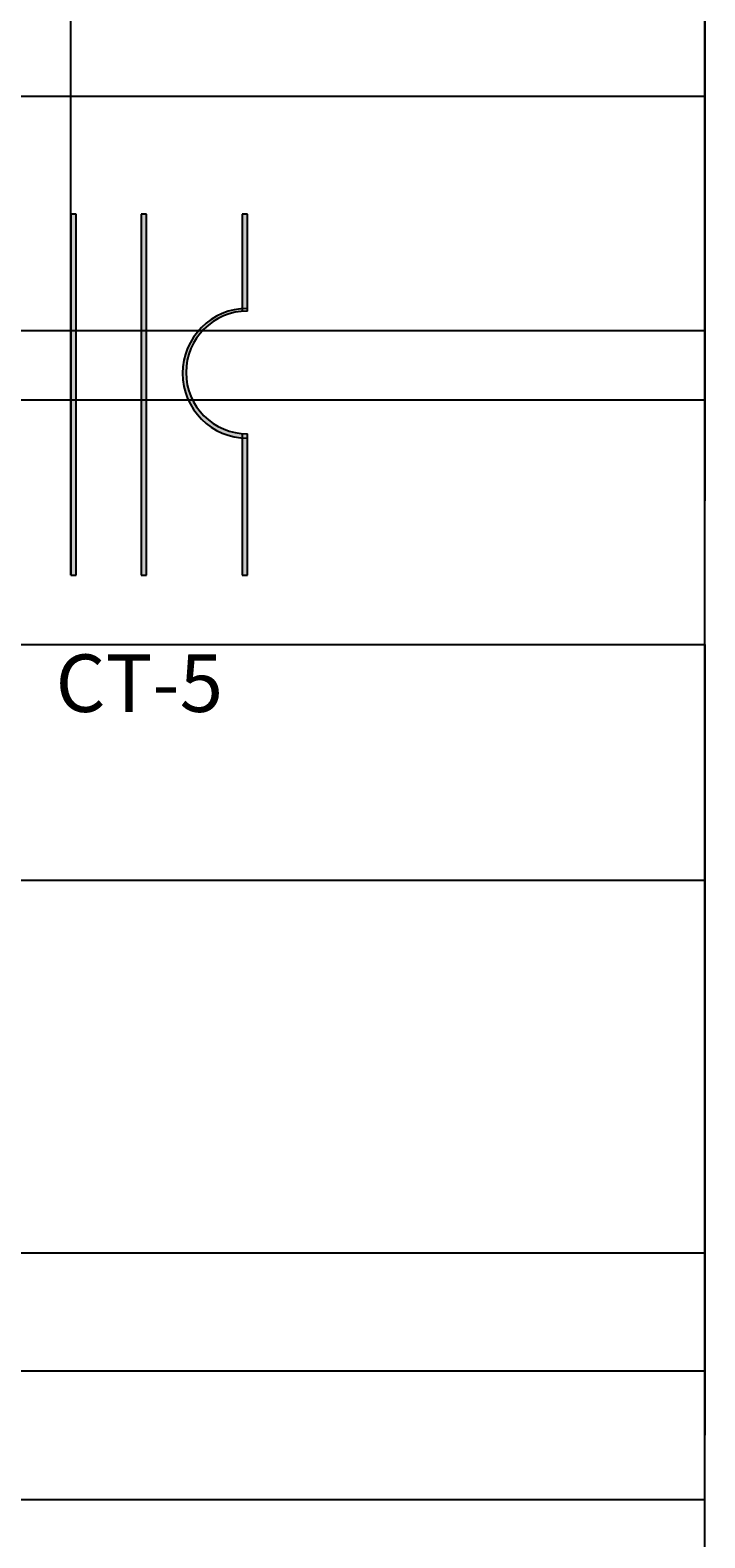
# Model space of a CAD drawing. Units: inches. Extents: x 35362 to 73946, y 43607 to 67532.
# Tile 134 of 134: x 71350 to 73946, y 55752 to 61547. Entities that reach past the tile are written whole.
import ezdxf

# ---------------------------------------------------------------- set-up
doc = ezdxf.new("R2010")
doc.units = ezdxf.units.IN
doc.header["$MEASUREMENT"] = 0
for name, color, linetype, lineweight in [('A-ANNO-DIMS', 2, 'Continuous', 18), ('E-ANNO-TEXT', 5, 'Continuous', 18), ('E-SYMB', 1, 'Continuous', 25), ('E-SYMB-PATT', 1, 'Continuous', 13)]:
    doc.layers.add(name, color=color, linetype=linetype, lineweight=lineweight)
doc.styles.get("Standard").update_dxf_attribs({"font": 'arial.ttf'})
doc.dimstyles.get("Standard").update_dxf_attribs({"dimtxt": 0.18, "dimasz": 0.18, "dimexe": 0.18, "dimexo": 0.0625, "dimgap": 0.09, "dimtad": 0, "dimtih": 1, "dimtoh": 1, "dimdec": 4, "dimzin": 0, "dimdsep": 46, "dimtxsty": 'Standard', "dimcen": 0.09, "dimadec": 0, "dimazin": 0, "dimtfac": 1, "dimtdec": 4, "dimtofl": 0, "dimtmove": 0, "dimatfit": 3, "dimfxl": 1, "dimtolj": 1, "dimtzin": 0, "dimarcsym": 0})

# ---------------------------------------------------------------- blocks, each defined once
blk = doc.blocks.new('CT-CORE')
for p, q in [((-0.0004610742907971, 1387.996120092102), (-0.0004610742907971, -5.34733626409e-05)), ((19.99953892572375, 1387.996120092102), (-0.0004610742907971, 1387.996120092102)), ((19.9995389257092, -5.34733626409e-05), (19.99953892572375, 1387.996120092102)), ((270.6681283192447, 1387.996120092102), (270.6681283192447, -5.34733626409e-05)), ((290.6681283192593, 1387.996120092102), (270.6681283192447, 1387.996120092102)), ((290.6681283192447, -5.34733626409e-05), (290.6681283192593, 1387.996120092102)), ((658.9826659540267, 1387.996120092102), (658.9826659540267, 1014.585417332389)), ((678.9826659540413, 1387.996120092102), (658.9826659540267, 1387.996120092102)), ((678.9826659540413, 1015.434583844784), (678.9826659540413, 1387.996120092102)), ((658.9826659540267, 544.3844491987692), (658.9826659540267, -5.34733626409e-05)), ((678.9826659540267, -5.34733626409e-05), (678.9826659540413, 543.5352826863744)), ((-0.0004610742907971, -5.34733626409e-05), (19.9995389257092, -5.34733626409e-05)), ((270.6681283192447, -5.34733626409e-05), (290.6681283192447, -5.34733626409e-05)), ((658.9826659540267, -5.34733626409e-05), (678.9826659540267, -5.34733626409e-05))]:
    blk.add_line(p, q)
blk.add_arc((678.9826659540267, 779.4849332655793), 235.9496505792049, 90, 270)
blk = doc.blocks.new('*D8')
at = {"layer": 'A-ANNO-DIMS', "color": 0, "lineweight": -2, "transparency": 16777216}
for p, q in [((66271.28651900003, 65771.51172800003), (73945.82566600003, 65771.51172800003)), ((73945.64566600005, 65771.33172800003), (73945.64566600005, 59737.03093663782)), ((73945.64566600005, 53702.36633900002), (73945.64566600005, 59736.66713036224)), ((72185.70816600003, 53702.18633900003), (73945.82566600003, 53702.18633900003))]:
    blk.add_line(p, q, dxfattribs=at)
at = {"layer": 'A-ANNO-DIMS', "color": 0, "transparency": 16777216}
for points in [[(73945.61566600006, 65771.33172800003), (73945.67566600005, 65771.33172800003), (73945.64566600005, 65771.51172800003)], [(73945.61566600006, 53702.36633900002), (73945.67566600005, 53702.36633900002), (73945.64566600005, 53702.18633900003)]]:
    blk.add_solid(points, dxfattribs=at)
at = {"layer": 'Defpoints', "color": 0, "transparency": 16777216}
for p in [(66271.22401900003, 65771.51172800003), (73945.64566600005, 65771.51172800003), (72185.64566600003, 53702.18633900003)]:
    blk.add_point(p, dxfattribs=at)
at = {"layer": 'A-ANNO-DIMS', "color": 0, "transparency": 16777216, "insert": (73945.64566600005, 59736.84903349999), "char_height": 0.18, "attachment_point": 5}
blk.add_mtext('\\A1;12069', dxfattribs=at)
blk = doc.blocks.new('*D10')
at = {"layer": 'A-ANNO-DIMS', "color": 0, "lineweight": -2, "transparency": 16777216}
for p, q in [((61240.96983600002, 59185.14395700003), (73945.82566600003, 59185.14395700003)), ((73945.64566600005, 59184.96395700003), (73945.64566600005, 56268.51827402935)), ((73945.64566600005, 53351.70866200003), (73945.64566600005, 56268.1543449707)), ((61240.96983600002, 53351.52866200003), (73945.82566600003, 53351.52866200003))]:
    blk.add_line(p, q, dxfattribs=at)
at = {"layer": 'A-ANNO-DIMS', "color": 0, "transparency": 16777216}
for points in [[(73945.61566600006, 59184.96395700003), (73945.67566600005, 59184.96395700003), (73945.64566600005, 59185.14395700003)], [(73945.61566600006, 53351.70866200003), (73945.67566600005, 53351.70866200003), (73945.64566600005, 53351.52866200003)]]:
    blk.add_solid(points, dxfattribs=at)
at = {"layer": 'Defpoints', "color": 0, "transparency": 16777216}
for p in [(61240.90733600002, 59185.14395700003), (61240.90733600002, 53351.52866200003), (73945.64566600005, 53351.52866200003)]:
    blk.add_point(p, dxfattribs=at)
at = {"layer": 'A-ANNO-DIMS', "color": 0, "transparency": 16777216, "insert": (73945.64566600005, 56268.33630949999), "char_height": 0.18, "attachment_point": 5}
blk.add_mtext('\\A1;5834', dxfattribs=at)
blk = doc.blocks.new('*D47')
at = {"layer": 'A-ANNO-DIMS', "color": 0, "lineweight": -2, "transparency": 16777216}
for p, q in [((50339.58680000003, 58279.98849500002), (73945.82566600003, 58279.98849500002)), ((73945.64566600005, 58279.80849500002), (73945.64566600005, 57564.17141502935)), ((73945.64566600005, 56848.17040600003), (73945.64566600005, 57563.80748597069)), ((50339.58680000003, 56847.99040600003), (73945.82566600003, 56847.99040600003))]:
    blk.add_line(p, q, dxfattribs=at)
at = {"layer": 'A-ANNO-DIMS', "color": 0, "transparency": 16777216}
for points in [[(73945.61566600006, 58279.80849500002), (73945.67566600005, 58279.80849500002), (73945.64566600005, 58279.98849500002)], [(73945.61566600006, 56848.17040600003), (73945.67566600005, 56848.17040600003), (73945.64566600005, 56847.99040600003)]]:
    blk.add_solid(points, dxfattribs=at)
at = {"layer": 'Defpoints', "color": 0, "transparency": 16777216}
for p in [(50339.52430000002, 58279.98849500002), (50339.52430000002, 56847.99040600003), (73945.64566600005, 56847.99040600003)]:
    blk.add_point(p, dxfattribs=at)
at = {"layer": 'A-ANNO-DIMS', "color": 0, "transparency": 16777216, "insert": (73945.64566600005, 57563.98945049999), "char_height": 0.18, "attachment_point": 5}
blk.add_mtext('\\A1;1432.0', dxfattribs=at)
blk = doc.blocks.new('*D50')
at = {"layer": 'A-ANNO-DIMS', "color": 0, "lineweight": -2, "transparency": 16777216}
for p, q in [((61657.28213900003, 56394.41825000003), (73945.82566600003, 56394.41825000003)), ((73945.64566600005, 56394.23825000003), (73945.64566600005, 56147.19337413782)), ((73945.64566600005, 55899.78469200003), (73945.64566600005, 56146.82956786224)), ((61657.28213900003, 55899.60469200002), (73945.82566600003, 55899.60469200002))]:
    blk.add_line(p, q, dxfattribs=at)
at = {"layer": 'A-ANNO-DIMS', "color": 0, "transparency": 16777216}
for points in [[(73945.61566600006, 56394.23825000003), (73945.67566600005, 56394.23825000003), (73945.64566600005, 56394.41825000003)], [(73945.61566600006, 55899.78469200003), (73945.67566600005, 55899.78469200003), (73945.64566600005, 55899.60469200002)]]:
    blk.add_solid(points, dxfattribs=at)
at = {"layer": 'Defpoints', "color": 0, "transparency": 16777216}
for p in [(61657.21963900003, 56394.41825000003), (61657.21963900003, 55899.60469200002), (73945.64566600005, 55899.60469200002)]:
    blk.add_point(p, dxfattribs=at)
at = {"layer": 'A-ANNO-DIMS', "color": 0, "transparency": 16777216, "insert": (73945.64566600005, 56147.01147099999), "char_height": 0.18, "attachment_point": 5}
blk.add_mtext('\\A1;494.8', dxfattribs=at)
blk = doc.blocks.new('*D66')
at = {"layer": 'A-ANNO-DIMS', "color": 0, "lineweight": -2, "transparency": 16777216}
for p, q in [((67326.70224100004, 64127.44160800003), (73945.82566600003, 64127.44160800003)), ((73945.64566600005, 64127.26160800003), (73945.64566600005, 62710.54579452936)), ((73945.64566600005, 61293.46605200003), (73945.64566600005, 62710.1818654707)), ((67326.70224100004, 61293.28605200003), (73945.82566600003, 61293.28605200003))]:
    blk.add_line(p, q, dxfattribs=at)
at = {"layer": 'A-ANNO-DIMS', "color": 0, "transparency": 16777216}
for points in [[(73945.61566600006, 64127.26160800003), (73945.67566600005, 64127.26160800003), (73945.64566600005, 64127.44160800003)], [(73945.61566600006, 61293.46605200003), (73945.67566600005, 61293.46605200003), (73945.64566600005, 61293.28605200003)]]:
    blk.add_solid(points, dxfattribs=at)
at = {"layer": 'Defpoints', "color": 0, "transparency": 16777216}
for p in [(67326.63974100004, 64127.44160800003), (73945.64566600005, 64127.44160800003), (67326.63974100004, 61293.28605200003)]:
    blk.add_point(p, dxfattribs=at)
at = {"layer": 'A-ANNO-DIMS', "color": 0, "transparency": 16777216, "insert": (73945.64566600005, 62710.36383), "char_height": 0.18, "attachment_point": 5}
blk.add_mtext('\\A1;2834.2', dxfattribs=at)
blk = doc.blocks.new('*D69')
at = {"layer": 'A-ANNO-DIMS', "color": 0, "lineweight": -2, "transparency": 16777216}
for p, q in [((68320.870762, 60122.408832), (68320.870762, 67531.691728)), ((68321.050762, 67531.51172799998), (69913.30289879469, 67531.51172799998)), ((71506.482539, 67531.51172799998), (69914.23040220531, 67531.51172799998)), ((71506.662539, 59451.647447), (71506.662539, 67531.691728))]:
    blk.add_line(p, q, dxfattribs=at)
at = {"layer": 'A-ANNO-DIMS', "color": 0, "transparency": 16777216}
for points in [[(68321.050762, 67531.541728), (68321.050762, 67531.481728), (68320.870762, 67531.51172799998)], [(71506.482539, 67531.541728), (71506.482539, 67531.481728), (71506.662539, 67531.51172799998)]]:
    blk.add_solid(points, dxfattribs=at)
at = {"layer": 'Defpoints', "color": 0, "transparency": 16777216}
for p in [(71506.662539, 67531.51172799998), (68320.870762, 60122.346332), (71506.662539, 59451.584947)]:
    blk.add_point(p, dxfattribs=at)
at = {"layer": 'A-ANNO-DIMS', "color": 0, "transparency": 16777216, "insert": (69913.76665050001, 67531.51172799998), "char_height": 0.18, "attachment_point": 5}
blk.add_mtext('\\A1;3185.8', dxfattribs=at)
blk = doc.blocks.new('*D70')
at = {"layer": 'A-ANNO-DIMS', "color": 0, "lineweight": -2, "transparency": 16777216}
for p, q in [((60785.27513900002, 64923.75242000003), (73945.82566600003, 64923.75242000003)), ((73945.64566600005, 64923.57242000003), (73945.64566600005, 62054.63015302935)), ((73945.64566600005, 59185.32395700003), (73945.64566600005, 62054.26622397069)), ((61240.96983600002, 59185.14395700003), (73945.82566600003, 59185.14395700003))]:
    blk.add_line(p, q, dxfattribs=at)
at = {"layer": 'A-ANNO-DIMS', "color": 0, "transparency": 16777216}
for points in [[(73945.61566600006, 64923.57242000003), (73945.67566600005, 64923.57242000003), (73945.64566600005, 64923.75242000003)], [(73945.61566600006, 59185.32395700003), (73945.67566600005, 59185.32395700003), (73945.64566600005, 59185.14395700003)]]:
    blk.add_solid(points, dxfattribs=at)
at = {"layer": 'Defpoints', "color": 0, "transparency": 16777216}
for p in [(60785.21263900002, 64923.75242000003), (73945.64566600005, 64923.75242000003), (61240.90733600002, 59185.14395700003)]:
    blk.add_point(p, dxfattribs=at)
at = {"layer": 'A-ANNO-DIMS', "color": 0, "transparency": 16777216, "insert": (73945.64566600005, 62054.44818849999), "char_height": 0.18, "attachment_point": 5}
blk.add_mtext('\\A1;5738.6', dxfattribs=at)
blk = doc.blocks.new('*D71')
at = {"layer": 'A-ANNO-DIMS', "color": 0, "lineweight": -2, "transparency": 16777216}
for p, q in [((63159.24181700003, 64828.55626700002), (73945.82566600003, 64828.55626700002)), ((73945.64566600005, 64828.37626700002), (73945.64566600005, 62007.03207652936)), ((73945.64566600005, 59185.32395700003), (73945.64566600005, 62006.6681474707)), ((61240.96983600002, 59185.14395700003), (73945.82566600003, 59185.14395700003))]:
    blk.add_line(p, q, dxfattribs=at)
at = {"layer": 'A-ANNO-DIMS', "color": 0, "transparency": 16777216}
for points in [[(73945.61566600006, 64828.37626700002), (73945.67566600005, 64828.37626700002), (73945.64566600005, 64828.55626700002)], [(73945.61566600006, 59185.32395700003), (73945.67566600005, 59185.32395700003), (73945.64566600005, 59185.14395700003)]]:
    blk.add_solid(points, dxfattribs=at)
at = {"layer": 'Defpoints', "color": 0, "transparency": 16777216}
for p in [(63159.17931700003, 64828.55626700002), (73945.64566600005, 64828.55626700002), (61240.90733600002, 59185.14395700003)]:
    blk.add_point(p, dxfattribs=at)
at = {"layer": 'A-ANNO-DIMS', "color": 0, "transparency": 16777216, "insert": (73945.64566600005, 62006.85011199999), "char_height": 0.18, "attachment_point": 5}
blk.add_mtext('\\A1;5643.4', dxfattribs=at)
blk = doc.blocks.new('*D113')
at = {"layer": 'A-ANNO-DIMS', "color": 0, "lineweight": -2, "transparency": 16777216}
for p, q in [((53526.13474100003, 60391.71935800003), (73945.82566600003, 60391.71935800003)), ((73945.64566600005, 60391.53935800003), (73945.64566600005, 60259.19182863781)), ((73945.64566600005, 60126.48049300003), (73945.64566600005, 60258.82802236224)), ((53705.42262200003, 60126.30049300003), (73945.82566600003, 60126.30049300003))]:
    blk.add_line(p, q, dxfattribs=at)
at = {"layer": 'A-ANNO-DIMS', "color": 0, "transparency": 16777216}
for points in [[(73945.61566600006, 60391.53935800003), (73945.67566600005, 60391.53935800003), (73945.64566600005, 60391.71935800003)], [(73945.61566600006, 60126.48049300003), (73945.67566600005, 60126.48049300003), (73945.64566600005, 60126.30049300003)]]:
    blk.add_solid(points, dxfattribs=at)
at = {"layer": 'Defpoints', "color": 0, "transparency": 16777216}
for p in [(53526.07224100003, 60391.71935800003), (73945.64566600005, 60391.71935800003), (53705.36012200003, 60126.30049300003)]:
    blk.add_point(p, dxfattribs=at)
at = {"layer": 'A-ANNO-DIMS', "color": 0, "transparency": 16777216, "insert": (73945.64566600005, 60259.00992549999), "char_height": 0.18, "attachment_point": 5}
blk.add_mtext('\\A1;265.4', dxfattribs=at)

msp = doc.modelspace()

# ---------------------------------------------------------------- hatches: boundary and pattern name
at = {"layer": 'E-SYMB-PATT'}
h = msp.add_hatch(color=256, dxfattribs=at)
h.dxf.hatch_style = 1
h.paths.add_polyline_path([(71526.66253892572, 60839.5811200921), (71506.66253892571, 60839.5811200921), (71506.66253892571, 59451.58494652663), (71526.6625389257, 59451.58494652663)])
h = msp.add_hatch(color=256, dxfattribs=at)
h.dxf.hatch_style = 1
h.paths.add_polyline_path([(71797.33112831926, 60839.5811200921), (71777.33112831925, 60839.5811200921), (71777.33112831925, 59451.58494652663), (71797.33112831925, 59451.58494652663)])
h = msp.add_hatch(color=256, dxfattribs=at)
h.dxf.hatch_style = 1
h.paths.add_polyline_path([(72185.64566595404, 59995.12028268637, -0.0212196039209565), (72165.64566595403, 59995.96944919876), (72165.64566595403, 59979.09653472976, 0.0200709024740955), (72185.64566595404, 59978.29337508506)])
h.paths.add_polyline_path([(72185.64566595404, 59978.29337508506, -0.0200709024740953), (72165.64566595403, 59979.09653472976), (72165.64566595403, 59451.58494652663), (72185.64566595403, 59451.58494652663)])
h.paths.add_polyline_path([(72185.64566595404, 60839.5811200921), (72165.64566595403, 60839.5811200921), (72165.64566595403, 60476.32636596064, -0.0200709024740959), (72185.64566595404, 60477.12952560534)])
h.paths.add_polyline_path([(72185.64566595404, 60477.12952560534, 0.020070902474096), (72165.64566595403, 60476.32636596063), (72165.64566595403, 60466.17041733239, -0.0212196039209564), (72185.64566595404, 60467.01958384478)])
h = msp.add_hatch(color=256, dxfattribs=at)
h.dxf.hatch_style = 1
h.paths.add_polyline_path([(72165.64566595403, 60466.17041733239), (72165.64566595403, 60476.32636596064, 0.3908929169039177), (71936.22759069389, 60227.7114503452, 0.3908929169039177), (72165.64566595403, 59979.09653472976), (72165.64566595403, 59995.96944919876, -0.389569854577291), (71949.69601537482, 60231.06993326558, -0.389569854577291)])

# ---------------------------------------------------------------- linework, layer by layer
at = {"layer": 'E-SYMB'}
msp.add_arc((72185.64566595403, 60227.7114503452), 249.4180752601387, 90, 270, dxfattribs=at)

# ---------------------------------------------------------------- block references
msp.add_blockref('CT-CORE', (71506.663, 59451.58499999999), dxfattribs=at)

# ---------------------------------------------------------------- texts
at = {"layer": 'E-ANNO-TEXT'}
msp.add_text('CT-5', height=220.8659825270206, dxfattribs=at).set_placement((71447.68333186794, 58926.23261734448))

# ---------------------------------------------------------------- dimensions: what is measured, and where the dimension line sits
at = {"layer": 'A-ANNO-DIMS'}
dim = msp.add_linear_dim(base=(71506.662539, 67531.51172799998), p1=(68320.870762, 60122.346332), p2=(71506.662539, 59451.584947), dimstyle='Standard', override={"dimdec": 1, "dimlfac": 1, "dimrnd": 0, "dimzin": 0, "dimdsep": 46, "dimlunit": 2}, dxfattribs=at)
dim.commit()
dim.dimension.update_dxf_attribs({"geometry": '*D69', "text_midpoint": (69913.76665050001, 67531.51172799998)})
for base, p1, p2, override, picture, middle in [((73945.64566600005, 65771.51172800003), (72185.645666, 53702.186339), (66271.224019, 65771.51172799998), {"dimdec": 0, "dimlfac": 1, "dimrnd": 0, "dimzin": 0, "dimdsep": 46, "dimlunit": 2}, '*D8', (73945.64566600005, 59736.84903349999)), ((73945.64566600005, 64923.75242000003), (61240.907336, 59185.14395699999), (60785.21263899999, 64923.75241999999), {"dimdec": 1, "dimlfac": 1, "dimrnd": 0, "dimzin": 0, "dimdsep": 46, "dimlunit": 2}, '*D70', (73945.64566600005, 62054.44818849999)), ((73945.64566600005, 64828.55626700002), (61240.907336, 59185.14395699999), (63159.179317, 64828.556267), {"dimdec": 1, "dimlfac": 1, "dimrnd": 0, "dimzin": 0, "dimdsep": 46, "dimlunit": 2}, '*D71', (73945.64566600005, 62006.85011199999)), ((73945.64566600005, 64127.44160800003), (67326.639741, 61293.286052), (67326.639741, 64127.44160799999), {"dimdec": 1, "dimlfac": 1, "dimrnd": 0, "dimzin": 0, "dimdsep": 46, "dimlunit": 2}, '*D66', (73945.64566600005, 62710.36383)), ((73945.64566600005, 60391.71935800003), (53705.36012199999, 60126.300493), (53526.072241, 60391.719358), {"dimdec": 1, "dimlfac": 1, "dimrnd": 0, "dimzin": 0, "dimdsep": 46, "dimlunit": 2}, '*D113', (73945.64566600005, 60259.00992549999)), ((73945.64566600005, 53351.52866200003), (61240.907336, 59185.14395699999), (61240.907336, 53351.52866199999), {"dimdec": 0, "dimlfac": 1, "dimrnd": 0, "dimzin": 0, "dimdsep": 46, "dimlunit": 2}, '*D10', (73945.64566600005, 56268.33630949999)), ((73945.64566600005, 56847.99040600003), (50339.5243, 58279.988495), (50339.5243, 56847.99040599999), {"dimdec": 1, "dimlfac": 1, "dimrnd": 0, "dimzin": 0, "dimdsep": 46, "dimlunit": 2}, '*D47', (73945.64566600005, 57563.98945049999)), ((73945.64566600005, 55899.60469200002), (61657.219639, 56394.41825), (61657.219639, 55899.604692), {"dimdec": 1, "dimlfac": 1, "dimrnd": 0, "dimzin": 0, "dimdsep": 46, "dimlunit": 2}, '*D50', (73945.64566600005, 56147.01147099999))]:
    dim = msp.add_linear_dim(base=base, p1=p1, p2=p2, angle=90, dimstyle='Standard', override=override, dxfattribs=at)
    dim.commit()
    dim.dimension.update_dxf_attribs({"geometry": picture, "text_midpoint": middle})

doc.saveas('drawing.dxf')
